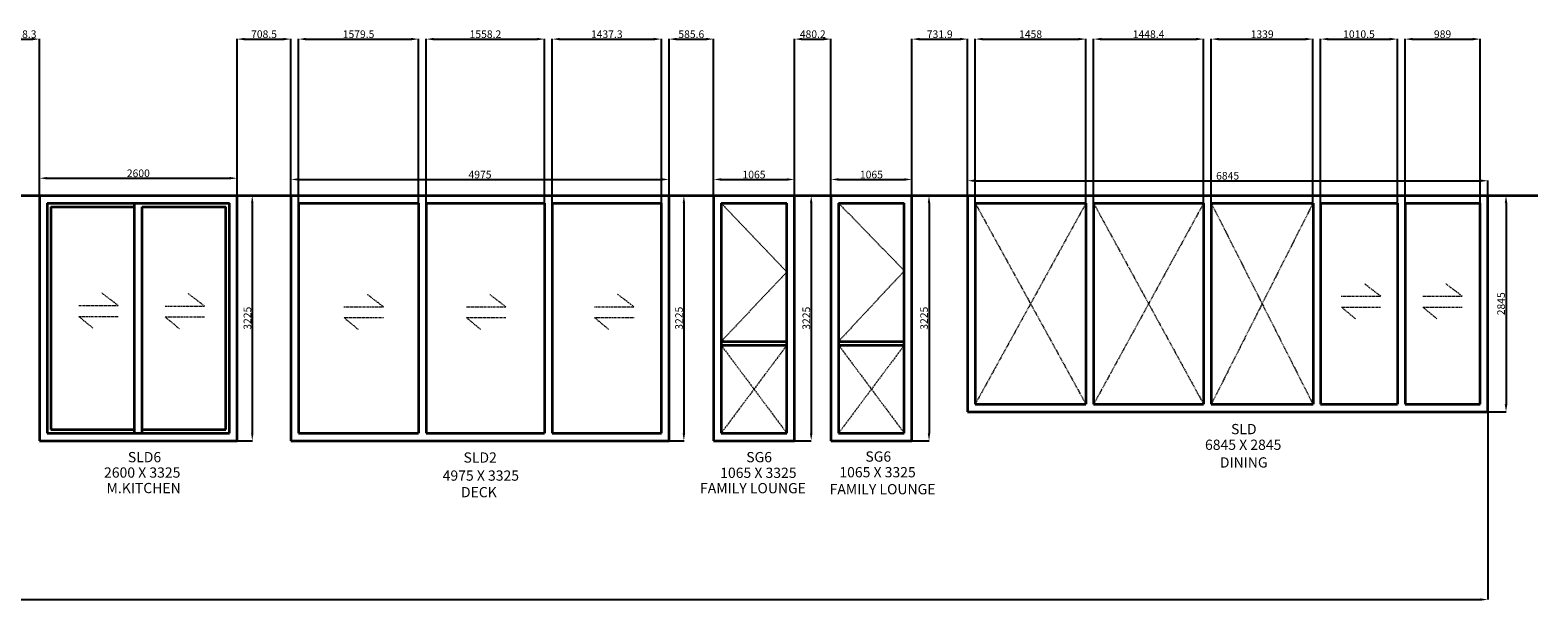
# Model space of a CAD drawing. Units: millimetres. Extents: x -850 to 42148, y -7352 to 4589.
# Tile 4 of 4: x 22310 to 42148, y -2915 to 4589. Entities that reach past the tile are written whole.
import ezdxf

# ---------------------------------------------------------------- set-up
doc = ezdxf.new("R2010")
doc.units = ezdxf.units.MM
doc.linetypes.add('DASHED', pattern=[19.05, 12.7, -6.35])
for name, color, linetype, lineweight in [('A-ANNO-DIMS', 2, 'Continuous', 18), ('A-ANNO-TEXT', 7, 'Continuous', 18), ('A-GLAZ', 4, 'Continuous', 35), ('A-GLAZ-OPNG', 4, 'DASHED', 18)]:
    doc.layers.add(name, color=color, linetype=linetype, lineweight=lineweight)
doc.styles.get("Standard").update_dxf_attribs({"font": 'arial.ttf'})
doc.dimstyles.new('ISO-25', dxfattribs={"dimtxt": 100, "dimasz": 100, "dimexe": 1.25, "dimexo": 0.625, "dimtad": 1, "dimtxsty": 'Standard', "dimcen": 2.5, "dimadec": 0, "dimazin": 0, "dimtfac": 1, "dimtmove": 0, "dimatfit": 3, "dimfxl": 1, "dimarcsym": 0})

# ---------------------------------------------------------------- blocks, each defined once
blk = doc.blocks.new('*D19')
at = {"layer": 'A-ANNO-DIMS', "color": 0, "lineweight": -2, "transparency": 16777216}
for p, q in [((22433, 2415), (22433, 2644)), ((22533, 2642), (24933, 2642)), ((25033, 2415), (25033, 2644))]:
    blk.add_line(p, q, dxfattribs=at)
at = {"layer": 'A-ANNO-DIMS', "color": 0, "lineweight": 30, "transparency": 16777216}
for points in [[(22533, 2659), (22533, 2626), (22433, 2642)], [(24933, 2659), (24933, 2626), (25033, 2642)]]:
    blk.add_solid(points, dxfattribs=at)
at = {"layer": 'Defpoints', "color": 0, "lineweight": 30, "transparency": 16777216}
for p in [(25033, 2642), (22433, 2414), (25033, 2414)]:
    blk.add_point(p, dxfattribs=at)
at = {"layer": 'A-ANNO-DIMS', "color": 0, "transparency": 16777216, "insert": (23733, 2694), "char_height": 100, "attachment_point": 5}
blk.add_mtext('2600', dxfattribs=at)
blk = doc.blocks.new('*D20')
at = {"layer": 'A-ANNO-DIMS', "color": 0, "lineweight": -2, "transparency": 16777216}
for p, q in [((25033, 2414), (25234, 2414)), ((25232, 2314), (25232, -711)), ((25033, -811), (25234, -811))]:
    blk.add_line(p, q, dxfattribs=at)
at = {"layer": 'A-ANNO-DIMS', "color": 0, "lineweight": 30, "transparency": 16777216}
for points in [[(25216, 2314), (25249, 2314), (25232, 2414)], [(25216, -711), (25249, -711), (25232, -811)]]:
    blk.add_solid(points, dxfattribs=at)
at = {"layer": 'Defpoints', "color": 0, "lineweight": 30, "transparency": 16777216}
for p in [(25033, 2414), (25033, -811), (25232, -811)]:
    blk.add_point(p, dxfattribs=at)
at = {"layer": 'A-ANNO-DIMS', "color": 0, "transparency": 16777216, "insert": (25181, 801), "char_height": 100, "attachment_point": 5, "rotation": 90}
blk.add_mtext('3225', dxfattribs=at)
blk = doc.blocks.new('*D21')
at = {"layer": 'A-ANNO-DIMS', "color": 0, "lineweight": -2, "transparency": 16777216}
for p, q in [((25741, 2415), (25741, 2627)), ((25841, 2626), (30616, 2626)), ((30716, 2415), (30716, 2627))]:
    blk.add_line(p, q, dxfattribs=at)
at = {"layer": 'A-ANNO-DIMS', "color": 0, "lineweight": 30, "transparency": 16777216}
for points in [[(25841, 2642), (25841, 2609), (25741, 2626)], [(30616, 2642), (30616, 2609), (30716, 2626)]]:
    blk.add_solid(points, dxfattribs=at)
at = {"layer": 'Defpoints', "color": 0, "lineweight": 30, "transparency": 16777216}
for p in [(30716, 2626), (25741, 2414), (30716, 2414)]:
    blk.add_point(p, dxfattribs=at)
at = {"layer": 'A-ANNO-DIMS', "color": 0, "transparency": 16777216, "insert": (28229, 2677), "char_height": 100, "attachment_point": 5}
blk.add_mtext('4975', dxfattribs=at)
blk = doc.blocks.new('*D22')
at = {"layer": 'A-ANNO-DIMS', "color": 0, "lineweight": -2, "transparency": 16777216}
for p, q in [((30717, 2414), (30913, 2414)), ((30911, 2314), (30911, -711)), ((30717, -811), (30913, -811))]:
    blk.add_line(p, q, dxfattribs=at)
at = {"layer": 'A-ANNO-DIMS', "color": 0, "lineweight": 30, "transparency": 16777216}
for points in [[(30895, 2314), (30928, 2314), (30911, 2414)], [(30895, -711), (30928, -711), (30911, -811)]]:
    blk.add_solid(points, dxfattribs=at)
at = {"layer": 'Defpoints', "color": 0, "lineweight": 30, "transparency": 16777216}
for p in [(30716, 2414), (30716, -811), (30911, -811)]:
    blk.add_point(p, dxfattribs=at)
at = {"layer": 'A-ANNO-DIMS', "color": 0, "transparency": 16777216, "insert": (30860, 801), "char_height": 100, "attachment_point": 5, "rotation": 90}
blk.add_mtext('3225', dxfattribs=at)
blk = doc.blocks.new('*D23')
at = {"layer": 'A-ANNO-DIMS', "color": 0, "lineweight": -2, "transparency": 16777216}
for p, q in [((31302, 2415), (31302, 2627)), ((31402, 2626), (32267, 2626)), ((32367, 2415), (32367, 2627))]:
    blk.add_line(p, q, dxfattribs=at)
at = {"layer": 'A-ANNO-DIMS', "color": 0, "lineweight": 30, "transparency": 16777216}
for points in [[(31402, 2642), (31402, 2609), (31302, 2626)], [(32267, 2642), (32267, 2609), (32367, 2626)]]:
    blk.add_solid(points, dxfattribs=at)
at = {"layer": 'Defpoints', "color": 0, "lineweight": 30, "transparency": 16777216}
for p in [(32367, 2626), (31302, 2414), (32367, 2414)]:
    blk.add_point(p, dxfattribs=at)
at = {"layer": 'A-ANNO-DIMS', "color": 0, "transparency": 16777216, "insert": (31834, 2677), "char_height": 100, "attachment_point": 5}
blk.add_mtext('1065', dxfattribs=at)
blk = doc.blocks.new('*D24')
at = {"layer": 'A-ANNO-DIMS', "color": 0, "lineweight": -2, "transparency": 16777216}
for p, q in [((32367, 2414), (32588, 2414)), ((32587, 2314), (32587, -711)), ((32367, -811), (32588, -811))]:
    blk.add_line(p, q, dxfattribs=at)
at = {"layer": 'A-ANNO-DIMS', "color": 0, "lineweight": 30, "transparency": 16777216}
for points in [[(32570, 2314), (32603, 2314), (32587, 2414)], [(32570, -711), (32603, -711), (32587, -811)]]:
    blk.add_solid(points, dxfattribs=at)
at = {"layer": 'Defpoints', "color": 0, "lineweight": 30, "transparency": 16777216}
for p in [(32367, 2414), (32367, -811), (32587, -811)]:
    blk.add_point(p, dxfattribs=at)
at = {"layer": 'A-ANNO-DIMS', "color": 0, "transparency": 16777216, "insert": (32535, 801), "char_height": 100, "attachment_point": 5, "rotation": 90}
blk.add_mtext('3225', dxfattribs=at)
blk = doc.blocks.new('*D25')
at = {"layer": 'A-ANNO-DIMS', "color": 0, "lineweight": -2, "transparency": 16777216}
for p, q in [((32847, 2415), (32847, 2627)), ((32947, 2626), (33812, 2626)), ((33912, 2415), (33912, 2627))]:
    blk.add_line(p, q, dxfattribs=at)
at = {"layer": 'A-ANNO-DIMS', "color": 0, "lineweight": 30, "transparency": 16777216}
for points in [[(32947, 2642), (32947, 2609), (32847, 2626)], [(33812, 2642), (33812, 2609), (33912, 2626)]]:
    blk.add_solid(points, dxfattribs=at)
at = {"layer": 'Defpoints', "color": 0, "lineweight": 30, "transparency": 16777216}
for p in [(33912, 2626), (32847, 2414), (33912, 2414)]:
    blk.add_point(p, dxfattribs=at)
at = {"layer": 'A-ANNO-DIMS', "color": 0, "transparency": 16777216, "insert": (33379, 2677), "char_height": 100, "attachment_point": 5}
blk.add_mtext('1065', dxfattribs=at)
blk = doc.blocks.new('*D26')
at = {"layer": 'A-ANNO-DIMS', "color": 0, "lineweight": -2, "transparency": 16777216}
for p, q in [((33912, 2414), (34138, 2414)), ((34137, 2314), (34137, -711)), ((33912, -811), (34138, -811))]:
    blk.add_line(p, q, dxfattribs=at)
at = {"layer": 'A-ANNO-DIMS', "color": 0, "lineweight": 30, "transparency": 16777216}
for points in [[(34120, 2314), (34153, 2314), (34137, 2414)], [(34120, -711), (34153, -711), (34137, -811)]]:
    blk.add_solid(points, dxfattribs=at)
at = {"layer": 'Defpoints', "color": 0, "lineweight": 30, "transparency": 16777216}
for p in [(33912, 2414), (33912, -811), (34137, -811)]:
    blk.add_point(p, dxfattribs=at)
at = {"layer": 'A-ANNO-DIMS', "color": 0, "transparency": 16777216, "insert": (34085, 801), "char_height": 100, "attachment_point": 5, "rotation": 90}
blk.add_mtext('3225', dxfattribs=at)
blk = doc.blocks.new('*D27')
at = {"layer": 'A-ANNO-DIMS', "color": 0, "lineweight": -2, "transparency": 16777216}
for p, q in [((34644, 2415), (34644, 2610)), ((34744, 2609), (41389, 2609)), ((41489, 2415), (41489, 2610))]:
    blk.add_line(p, q, dxfattribs=at)
at = {"layer": 'A-ANNO-DIMS', "color": 0, "lineweight": 30, "transparency": 16777216}
for points in [[(34744, 2626), (34744, 2592), (34644, 2609)], [(41389, 2626), (41389, 2592), (41489, 2609)]]:
    blk.add_solid(points, dxfattribs=at)
at = {"layer": 'Defpoints', "color": 0, "lineweight": 30, "transparency": 16777216}
for p in [(41489, 2609), (34644, 2414), (41489, 2414)]:
    blk.add_point(p, dxfattribs=at)
at = {"layer": 'A-ANNO-DIMS', "color": 0, "transparency": 16777216, "insert": (38066, 2661), "char_height": 100, "attachment_point": 5}
blk.add_mtext('6845', dxfattribs=at)
blk = doc.blocks.new('*D28')
at = {"layer": 'A-ANNO-DIMS', "color": 0, "lineweight": -2, "transparency": 16777216}
for p, q in [((41489, 2414), (41730, 2414)), ((41729, 2314), (41729, -331)), ((41489, -431), (41730, -431))]:
    blk.add_line(p, q, dxfattribs=at)
at = {"layer": 'A-ANNO-DIMS', "color": 0, "lineweight": 30, "transparency": 16777216}
for points in [[(41712, 2314), (41746, 2314), (41729, 2414)], [(41712, -331), (41746, -331), (41729, -431)]]:
    blk.add_solid(points, dxfattribs=at)
at = {"layer": 'Defpoints', "color": 0, "lineweight": 30, "transparency": 16777216}
for p in [(41489, 2414), (41489, -431), (41729, -431)]:
    blk.add_point(p, dxfattribs=at)
at = {"layer": 'A-ANNO-DIMS', "color": 0, "transparency": 16777216, "insert": (41677, 991), "char_height": 100, "attachment_point": 5, "rotation": 90}
blk.add_mtext('2845', dxfattribs=at)
blk = doc.blocks.new('SYM-SLIDE-ARROW')
for p, q in [((2602, 903), (2388, 1066)), ((2084, 903), (2602, 903)), ((2085, 760), (2604, 760)), ((2085, 760), (2269, 607))]:
    blk.add_line(p, q)
blk = doc.blocks.new('*D60')
at = {"layer": 'A-ANNO-DIMS', "color": 0, "lineweight": -2, "transparency": 16777216}
for p, q in [((41489, -432), (41489, -2900)), ((1325, -812), (1325, -2900)), ((1425, -2899), (41389, -2899))]:
    blk.add_line(p, q, dxfattribs=at)
at = {"layer": 'A-ANNO-DIMS', "color": 0, "lineweight": 30, "transparency": 16777216}
for points in [[(1425, -2882), (1425, -2915), (1325, -2899)], [(41389, -2882), (41389, -2915), (41489, -2899)]]:
    blk.add_solid(points, dxfattribs=at)
at = {"layer": 'Defpoints', "color": 0, "lineweight": 30, "transparency": 16777216}
for p in [(41489, -431), (1325, -811), (41489, -2899)]:
    blk.add_point(p, dxfattribs=at)
at = {"layer": 'A-ANNO-DIMS', "color": 0, "transparency": 16777216, "insert": (21407, -2847), "char_height": 100, "attachment_point": 5}
blk.add_mtext('40164', dxfattribs=at)
blk = doc.blocks.new('*D69')
at = {"layer": 'A-ANNO-DIMS', "color": 0, "lineweight": -2, "transparency": 16777216}
for p, q in [((22014, 2415), (22014, 4473)), ((22114, 4471), (22333, 4471)), ((22433, 2415), (22433, 4473))]:
    blk.add_line(p, q, dxfattribs=at)
at = {"layer": 'A-ANNO-DIMS', "color": 0, "lineweight": 30, "transparency": 16777216}
for points in [[(22114, 4488), (22114, 4455), (22014, 4471)], [(22333, 4488), (22333, 4455), (22433, 4471)]]:
    blk.add_solid(points, dxfattribs=at)
at = {"layer": 'Defpoints', "color": 0, "lineweight": 30, "transparency": 16777216}
for p in [(22433, 4471), (22014, 2414), (22433, 2414)]:
    blk.add_point(p, dxfattribs=at)
at = {"layer": 'A-ANNO-DIMS', "color": 0, "transparency": 16777216, "insert": (22223, 4523), "char_height": 100, "attachment_point": 5}
blk.add_mtext('418.3', dxfattribs=at)
blk = doc.blocks.new('*D70')
at = {"layer": 'A-ANNO-DIMS', "color": 0, "lineweight": -2, "transparency": 16777216}
for p, q in [((25033, 2415), (25033, 4473)), ((25133, 4471), (25641, 4471)), ((25741, 2415), (25741, 4473))]:
    blk.add_line(p, q, dxfattribs=at)
at = {"layer": 'A-ANNO-DIMS', "color": 0, "lineweight": 30, "transparency": 16777216}
for points in [[(25133, 4488), (25133, 4455), (25033, 4471)], [(25641, 4488), (25641, 4455), (25741, 4471)]]:
    blk.add_solid(points, dxfattribs=at)
at = {"layer": 'Defpoints', "color": 0, "lineweight": 30, "transparency": 16777216}
for p in [(25741, 4471), (25033, 2414), (25741, 2414)]:
    blk.add_point(p, dxfattribs=at)
at = {"layer": 'A-ANNO-DIMS', "color": 0, "transparency": 16777216, "insert": (25387, 4523), "char_height": 100, "attachment_point": 5}
blk.add_mtext('708.5', dxfattribs=at)
blk = doc.blocks.new('*D71')
at = {"layer": 'A-ANNO-DIMS', "color": 0, "lineweight": -2, "transparency": 16777216}
for p, q in [((30716, 2415), (30716, 4473)), ((30816, 4471), (31202, 4471)), ((31302, 2415), (31302, 4473))]:
    blk.add_line(p, q, dxfattribs=at)
at = {"layer": 'A-ANNO-DIMS', "color": 0, "lineweight": 30, "transparency": 16777216}
for points in [[(30816, 4488), (30816, 4455), (30716, 4471)], [(31202, 4488), (31202, 4455), (31302, 4471)]]:
    blk.add_solid(points, dxfattribs=at)
at = {"layer": 'Defpoints', "color": 0, "lineweight": 30, "transparency": 16777216}
for p in [(31302, 4471), (30716, 2414), (31302, 2414)]:
    blk.add_point(p, dxfattribs=at)
at = {"layer": 'A-ANNO-DIMS', "color": 0, "transparency": 16777216, "insert": (31009, 4523), "char_height": 100, "attachment_point": 5}
blk.add_mtext('585.6', dxfattribs=at)
blk = doc.blocks.new('*D72')
at = {"layer": 'A-ANNO-DIMS', "color": 0, "lineweight": -2, "transparency": 16777216}
for p, q in [((32367, 2415), (32367, 4473)), ((32467, 4471), (32747, 4471)), ((32847, 2415), (32847, 4473))]:
    blk.add_line(p, q, dxfattribs=at)
at = {"layer": 'A-ANNO-DIMS', "color": 0, "lineweight": 30, "transparency": 16777216}
for points in [[(32467, 4488), (32467, 4455), (32367, 4471)], [(32747, 4488), (32747, 4455), (32847, 4471)]]:
    blk.add_solid(points, dxfattribs=at)
at = {"layer": 'Defpoints', "color": 0, "lineweight": 30, "transparency": 16777216}
for p in [(32847, 4471), (32367, 2414), (32847, 2414)]:
    blk.add_point(p, dxfattribs=at)
at = {"layer": 'A-ANNO-DIMS', "color": 0, "transparency": 16777216, "insert": (32607, 4523), "char_height": 100, "attachment_point": 5}
blk.add_mtext('480.2', dxfattribs=at)
blk = doc.blocks.new('*D73')
at = {"layer": 'A-ANNO-DIMS', "color": 0, "lineweight": -2, "transparency": 16777216}
for p, q in [((33912, 2415), (33912, 4473)), ((34012, 4471), (34544, 4471)), ((34644, 2415), (34644, 4473))]:
    blk.add_line(p, q, dxfattribs=at)
at = {"layer": 'A-ANNO-DIMS', "color": 0, "lineweight": 30, "transparency": 16777216}
for points in [[(34012, 4488), (34012, 4455), (33912, 4471)], [(34544, 4488), (34544, 4455), (34644, 4471)]]:
    blk.add_solid(points, dxfattribs=at)
at = {"layer": 'Defpoints', "color": 0, "lineweight": 30, "transparency": 16777216}
for p in [(34644, 4471), (33912, 2414), (34644, 2414)]:
    blk.add_point(p, dxfattribs=at)
at = {"layer": 'A-ANNO-DIMS', "color": 0, "transparency": 16777216, "insert": (34278, 4523), "char_height": 100, "attachment_point": 5}
blk.add_mtext('731.9', dxfattribs=at)
blk = doc.blocks.new('*D75')
at = {"layer": 'A-ANNO-DIMS', "color": 0, "lineweight": -2, "transparency": 16777216}
for p, q in [((34744, 2315), (34744, 4473)), ((34844, 4471), (36102, 4471)), ((36202, 2315), (36202, 4473))]:
    blk.add_line(p, q, dxfattribs=at)
at = {"layer": 'A-ANNO-DIMS', "color": 0, "lineweight": 30, "transparency": 16777216}
for points in [[(34844, 4488), (34844, 4455), (34744, 4471)], [(36102, 4488), (36102, 4455), (36202, 4471)]]:
    blk.add_solid(points, dxfattribs=at)
at = {"layer": 'Defpoints', "color": 0, "lineweight": 30, "transparency": 16777216}
for p in [(36202, 4471), (34744, 2314), (36202, 2314)]:
    blk.add_point(p, dxfattribs=at)
at = {"layer": 'A-ANNO-DIMS', "color": 0, "transparency": 16777216, "insert": (35473, 4523), "char_height": 100, "attachment_point": 5}
blk.add_mtext('1458', dxfattribs=at)
blk = doc.blocks.new('*D76')
at = {"layer": 'A-ANNO-DIMS', "color": 0, "lineweight": -2, "transparency": 16777216}
for p, q in [((36302, 2315), (36302, 4473)), ((36402, 4471), (37650, 4471)), ((37750, 2315), (37750, 4473))]:
    blk.add_line(p, q, dxfattribs=at)
at = {"layer": 'A-ANNO-DIMS', "color": 0, "lineweight": 30, "transparency": 16777216}
for points in [[(36402, 4488), (36402, 4455), (36302, 4471)], [(37650, 4488), (37650, 4455), (37750, 4471)]]:
    blk.add_solid(points, dxfattribs=at)
at = {"layer": 'Defpoints', "color": 0, "lineweight": 30, "transparency": 16777216}
for p in [(37750, 4471), (36302, 2314), (37750, 2314)]:
    blk.add_point(p, dxfattribs=at)
at = {"layer": 'A-ANNO-DIMS', "color": 0, "transparency": 16777216, "insert": (37026, 4523), "char_height": 100, "attachment_point": 5}
blk.add_mtext('1448.4', dxfattribs=at)
blk = doc.blocks.new('*D77')
at = {"layer": 'A-ANNO-DIMS', "color": 0, "lineweight": -2, "transparency": 16777216}
for p, q in [((37850, 2315), (37850, 4473)), ((37950, 4471), (39089, 4471)), ((39189, 2315), (39189, 4473))]:
    blk.add_line(p, q, dxfattribs=at)
at = {"layer": 'A-ANNO-DIMS', "color": 0, "lineweight": 30, "transparency": 16777216}
for points in [[(37950, 4488), (37950, 4455), (37850, 4471)], [(39089, 4488), (39089, 4455), (39189, 4471)]]:
    blk.add_solid(points, dxfattribs=at)
at = {"layer": 'Defpoints', "color": 0, "lineweight": 30, "transparency": 16777216}
for p in [(39189, 4471), (37850, 2314), (39189, 2314)]:
    blk.add_point(p, dxfattribs=at)
at = {"layer": 'A-ANNO-DIMS', "color": 0, "transparency": 16777216, "insert": (38520, 4523), "char_height": 100, "attachment_point": 5}
blk.add_mtext('1339', dxfattribs=at)
blk = doc.blocks.new('*D78')
at = {"layer": 'A-ANNO-DIMS', "color": 0, "lineweight": -2, "transparency": 16777216}
for p, q in [((39289, 2315), (39289, 4473)), ((39389, 4471), (40200, 4471)), ((40300, 2315), (40300, 4473))]:
    blk.add_line(p, q, dxfattribs=at)
at = {"layer": 'A-ANNO-DIMS', "color": 0, "lineweight": 30, "transparency": 16777216}
for points in [[(39389, 4488), (39389, 4455), (39289, 4471)], [(40200, 4488), (40200, 4455), (40300, 4471)]]:
    blk.add_solid(points, dxfattribs=at)
at = {"layer": 'Defpoints', "color": 0, "lineweight": 30, "transparency": 16777216}
for p in [(40300, 4471), (39289, 2314), (40300, 2314)]:
    blk.add_point(p, dxfattribs=at)
at = {"layer": 'A-ANNO-DIMS', "color": 0, "transparency": 16777216, "insert": (39794, 4523), "char_height": 100, "attachment_point": 5}
blk.add_mtext('1010.5', dxfattribs=at)
blk = doc.blocks.new('*D79')
at = {"layer": 'A-ANNO-DIMS', "color": 0, "lineweight": -2, "transparency": 16777216}
for p, q in [((40400, 2315), (40400, 4473)), ((40500, 4471), (41289, 4471)), ((41389, 2315), (41389, 4473))]:
    blk.add_line(p, q, dxfattribs=at)
at = {"layer": 'A-ANNO-DIMS', "color": 0, "lineweight": 30, "transparency": 16777216}
for points in [[(40500, 4488), (40500, 4455), (40400, 4471)], [(41289, 4488), (41289, 4455), (41389, 4471)]]:
    blk.add_solid(points, dxfattribs=at)
at = {"layer": 'Defpoints', "color": 0, "lineweight": 30, "transparency": 16777216}
for p in [(41389, 4471), (40400, 2314), (41389, 2314)]:
    blk.add_point(p, dxfattribs=at)
at = {"layer": 'A-ANNO-DIMS', "color": 0, "transparency": 16777216, "insert": (40894, 4523), "char_height": 100, "attachment_point": 5}
blk.add_mtext('989', dxfattribs=at)
blk = doc.blocks.new('*D80')
at = {"layer": 'A-ANNO-DIMS', "color": 0, "lineweight": -2, "transparency": 16777216}
for p, q in [((25841, 2315), (25841, 4473)), ((25941, 4471), (27321, 4471)), ((27421, 2315), (27421, 4473))]:
    blk.add_line(p, q, dxfattribs=at)
at = {"layer": 'A-ANNO-DIMS', "color": 0, "lineweight": 30, "transparency": 16777216}
for points in [[(25941, 4488), (25941, 4455), (25841, 4471)], [(27321, 4488), (27321, 4455), (27421, 4471)]]:
    blk.add_solid(points, dxfattribs=at)
at = {"layer": 'Defpoints', "color": 0, "lineweight": 30, "transparency": 16777216}
for p in [(27421, 4471), (25841, 2314), (27421, 2314)]:
    blk.add_point(p, dxfattribs=at)
at = {"layer": 'A-ANNO-DIMS', "color": 0, "transparency": 16777216, "insert": (26631, 4523), "char_height": 100, "attachment_point": 5}
blk.add_mtext('1579.5', dxfattribs=at)
blk = doc.blocks.new('*D81')
at = {"layer": 'A-ANNO-DIMS', "color": 0, "lineweight": -2, "transparency": 16777216}
for p, q in [((27521, 2315), (27521, 4473)), ((27621, 4471), (28979, 4471)), ((29079, 2315), (29079, 4473))]:
    blk.add_line(p, q, dxfattribs=at)
at = {"layer": 'A-ANNO-DIMS', "color": 0, "lineweight": 30, "transparency": 16777216}
for points in [[(27621, 4488), (27621, 4455), (27521, 4471)], [(28979, 4488), (28979, 4455), (29079, 4471)]]:
    blk.add_solid(points, dxfattribs=at)
at = {"layer": 'Defpoints', "color": 0, "lineweight": 30, "transparency": 16777216}
for p in [(29079, 4471), (27521, 2314), (29079, 2314)]:
    blk.add_point(p, dxfattribs=at)
at = {"layer": 'A-ANNO-DIMS', "color": 0, "transparency": 16777216, "insert": (28300, 4523), "char_height": 100, "attachment_point": 5}
blk.add_mtext('1558.2', dxfattribs=at)
blk = doc.blocks.new('*D82')
at = {"layer": 'A-ANNO-DIMS', "color": 0, "lineweight": -2, "transparency": 16777216}
for p, q in [((29179, 2315), (29179, 4473)), ((29279, 4471), (30516, 4471)), ((30616, 2315), (30616, 4473))]:
    blk.add_line(p, q, dxfattribs=at)
at = {"layer": 'A-ANNO-DIMS', "color": 0, "lineweight": 30, "transparency": 16777216}
for points in [[(29279, 4488), (29279, 4455), (29179, 4471)], [(30516, 4488), (30516, 4455), (30616, 4471)]]:
    blk.add_solid(points, dxfattribs=at)
at = {"layer": 'Defpoints', "color": 0, "lineweight": 30, "transparency": 16777216}
for p in [(30616, 4471), (29179, 2314), (30616, 2314)]:
    blk.add_point(p, dxfattribs=at)
at = {"layer": 'A-ANNO-DIMS', "color": 0, "transparency": 16777216, "insert": (29897, 4523), "char_height": 100, "attachment_point": 5}
blk.add_mtext('1437.3', dxfattribs=at)

msp = doc.modelspace()

# ---------------------------------------------------------------- linework, layer by layer
at = {"layer": 'A-GLAZ'}
for p, q in [((15219.457, 2413.876), (42147.613, 2413.876)), ((22432.638, 2413.876), (22432.638, -811.124)), ((25032.638, -811.124), (25032.638, 2413.876)), ((25741.095, 2413.876), (25741.095, -811.124)), ((30716.095, -811.124), (30716.095, 2413.876)), ((31301.669, 2413.876), (31301.669, -811.124)), ((32366.669, -811.124), (32366.669, 2413.876)), ((32846.844, 2413.876), (32846.844, -811.124)), ((33911.844, -811.124), (33911.844, 2413.876)), ((34643.766, 2413.876), (34643.766, -431.124)), ((41488.766, -431.124), (41488.766, 2413.876)), ((22532.638, 2313.876), (24932.638, 2313.876)), ((22532.638, 2313.876), (22532.638, -711.124)), ((22582.638, 2263.876), (22582.638, -661.124)), ((22582.638, 2263.876), (23682.638, 2263.876)), ((23682.638, -711.124), (23682.638, 2313.876)), ((23782.638, -711.124), (23782.638, 2263.876)), ((23782.638, 2263.876), (24882.638, 2263.876)), ((24882.638, -661.124), (24882.638, 2263.876)), ((24932.638, -711.124), (24932.638, 2313.876)), ((25841.095, 2313.876), (27420.566, 2313.876)), ((25841.095, 2313.876), (25841.095, -711.124)), ((27420.566, 2313.876), (27420.566, -711.124)), ((27520.566, 2313.876), (27520.566, -711.124)), ((27520.566, 2313.876), (29078.754, 2313.876)), ((29078.754, 2313.876), (29078.754, -711.124)), ((29178.754, 2313.876), (29178.754, -711.124)), ((29178.754, 2313.876), (30616.095, 2313.876)), ((30616.095, -711.124), (30616.095, 2313.876)), ((31401.669, 2313.876), (32266.669, 2313.876)), ((31401.669, 2313.876), (31401.669, -711.124)), ((32266.669, -711.124), (32266.669, 2313.876)), ((32946.844, 2313.876), (32946.844, -711.124)), ((32946.844, 2313.876), (33811.844, 2313.876)), ((33811.844, -711.124), (33811.844, 2313.876)), ((34743.766, 2313.876), (34743.766, -331.124)), ((34743.766, 2313.876), (36201.908, 2313.876)), ((36201.908, 2313.876), (36201.908, -331.124)), ((36301.908, 2313.876), (36301.908, -331.124)), ((36301.908, 2313.876), (37750.325, 2313.876)), ((37750.325, 2313.876), (37750.325, -331.124)), ((37850.325, 2313.876), (37850.325, -331.124)), ((37850.325, 2313.876), (39189.258, 2313.876)), ((39189.258, 2313.876), (39189.258, -331.124)), ((39289.258, 2313.876), (39289.258, -331.124)), ((39289.258, 2313.876), (40299.738, 2313.876)), ((40299.738, 2313.876), (40299.738, -331.124)), ((40399.738, 2313.876), (40399.738, -331.124)), ((40399.738, 2313.876), (41388.766, 2313.876)), ((41388.766, -331.124), (41388.766, 2313.876)), ((31401.669, 496.763), (32266.669, 496.763)), ((31401.669, 446.763), (32266.669, 446.763)), ((32946.844, 496.763), (33811.844, 496.763)), ((32946.844, 446.763), (33811.844, 446.763)), ((34743.766, -331.124), (36201.908, -331.124)), ((36301.908, -331.124), (37750.325, -331.124)), ((37850.325, -331.124), (39189.258, -331.124)), ((39289.258, -331.124), (40299.738, -331.124)), ((40399.738, -331.124), (41388.766, -331.124)), ((34643.766, -431.124), (41488.766, -431.124)), ((22532.638, -711.124), (24932.638, -711.124)), ((22582.638, -661.124), (23682.638, -661.124)), ((23782.638, -661.124), (24882.638, -661.124)), ((25841.095, -711.124), (27420.566, -711.124)), ((27520.566, -711.124), (29078.754, -711.124)), ((29178.754, -711.124), (30616.095, -711.124)), ((31401.669, -711.124), (32266.669, -711.124)), ((32946.844, -711.124), (33811.844, -711.124)), ((22432.638, -811.124), (25032.638, -811.124)), ((25741.095, -811.124), (30716.095, -811.124)), ((31301.669, -811.124), (32366.669, -811.124)), ((32846.844, -811.124), (33911.844, -811.124))]:
    msp.add_line(p, q, dxfattribs=at)
at = {"layer": 'A-GLAZ-OPNG'}
for p, q in [((31401.669, 2313.876), (32266.669, 1407.83)), ((32946.844, 2313.876), (33811.844, 1424.913)), ((34743.766, 2313.876), (36201.908, -331.124)), ((36201.908, 2313.876), (34743.766, -331.124)), ((36301.908, 2313.876), (37750.325, -331.124)), ((37750.325, 2313.876), (36301.908, -331.124)), ((37850.325, 2313.876), (39189.258, -331.124)), ((39189.258, 2313.876), (37850.325, -331.124)), ((32266.669, 1407.83), (31401.669, 496.763)), ((33811.844, 1424.913), (32946.844, 496.763)), ((31401.669, 446.763), (32266.669, -711.124)), ((32266.669, 446.763), (31401.669, -711.124)), ((32946.844, 446.763), (33811.844, -711.124)), ((33811.844, 446.763), (32946.844, -711.124))]:
    msp.add_line(p, q, dxfattribs=at)

# ---------------------------------------------------------------- block references
for p in [(37477.561, 188.014), (38549.338, 188.014), (20865.848, 65.004), (22001.521, 58.408), (24354.924, 48.946), (25965.905, 48.946), (27652.064, 48.946)]:
    msp.add_blockref('SYM-SLIDE-ARROW', p, dxfattribs=at)

# ---------------------------------------------------------------- texts
at = {"layer": 'A-ANNO-TEXT'}
for s, height, p in [('SLD', 134.8889, (38110.859, -724.457)), ('6845 X 2845', 134.88886, (37768.085, -930.294)), ('SLD6', 134.8889, (23595.216, -1093.156)), ('SLD2', 134.8889, (28011.861, -1098.41)), ('SG6', 134.8889, (31732.015, -1093.156)), ('SG6', 134.8889, (33299.837, -1085.573)), ('2600 X 3325', 134.88886, (23281.786, -1295.736)), ('1065 X 3325', 134.88886, (31389.242, -1298.993)), ('1065 X 3325', 134.88886, (32957.063, -1291.41)), ('DINING', 134.8889, (37963.612, -1162.82)), ('M.KITCHEN', 134.8889, (23314.757, -1499.944)), ('4975 X 3325', 134.88886, (27737.454, -1335.769)), ('FAMILY LOUNGE', 134.88886, (31123.991, -1501.182)), ('FAMILY LOUNGE', 134.88886, (32829.121, -1514.704)), ('DECK', 134.8889, (27978.259, -1553.742))]:
    msp.add_text(s, height=height, dxfattribs=at).set_placement(p)

# ---------------------------------------------------------------- dimensions: what is measured, and where the dimension line sits
at = {"layer": 'A-ANNO-DIMS'}
for base, p1, p2, override, picture, middle in [((22432.638, 4471.376), (22014.328, 2413.876), (22432.638, 2413.876), {"dimdec": 1, "dimlfac": 1, "dimrnd": 0, "dimzin": 0, "dimdsep": 46, "dimlunit": 2}, '*D69', (22223.483, 4523.092)), ((25741.095, 4471.376), (25032.638, 2413.876), (25741.095, 2413.876), {"dimdec": 1, "dimlfac": 1, "dimrnd": 0, "dimzin": 0, "dimdsep": 46, "dimlunit": 2}, '*D70', (25386.867, 4523.058)), ((27420.566, 4471.376), (25841.095, 2313.876), (27420.566, 2313.876), {"dimdec": 1, "dimlfac": 1, "dimrnd": 0, "dimzin": 0, "dimdsep": 46, "dimlunit": 2}, '*D80', (26630.83, 4523.058)), ((29078.754, 4471.376), (27520.566, 2313.876), (29078.754, 2313.876), {"dimdec": 1, "dimlfac": 1, "dimrnd": 0, "dimzin": 0, "dimdsep": 46, "dimlunit": 2}, '*D81', (28299.66, 4523.058)), ((30616.095, 4471.376), (29178.754, 2313.876), (30616.095, 2313.876), {"dimdec": 1, "dimlfac": 1, "dimrnd": 0, "dimzin": 0, "dimdsep": 46, "dimlunit": 2}, '*D82', (29897.424, 4523.092)), ((31301.669, 4471.376), (30716.095, 2413.876), (31301.669, 2413.876), {"dimdec": 1, "dimlfac": 1, "dimrnd": 0, "dimzin": 0, "dimdsep": 46, "dimlunit": 2}, '*D71', (31008.882, 4523.058)), ((32846.844, 4471.376), (32366.669, 2413.876), (32846.844, 2413.876), {"dimdec": 1, "dimlfac": 1, "dimrnd": 0, "dimzin": 0, "dimdsep": 46, "dimlunit": 2}, '*D72', (32606.757, 4523.058)), ((34643.766, 4471.376), (33911.844, 2413.876), (34643.766, 2413.876), {"dimdec": 1, "dimlfac": 1, "dimrnd": 0, "dimzin": 0, "dimdsep": 46, "dimlunit": 2}, '*D73', (34277.805, 4523.092)), ((36201.908, 4471.376), (34743.766, 2313.876), (36201.908, 2313.876), {"dimdec": 0, "dimlfac": 1, "dimrnd": 0, "dimzin": 0, "dimdsep": 46, "dimlunit": 2}, '*D75', (35472.837, 4523.058)), ((37750.325, 4471.376), (36301.908, 2313.876), (37750.325, 2313.876), {"dimdec": 1, "dimlfac": 1, "dimrnd": 0, "dimzin": 0, "dimdsep": 46, "dimlunit": 2}, '*D76', (37026.117, 4523.058)), ((39189.258, 4471.376), (37850.325, 2313.876), (39189.258, 2313.876), {"dimdec": 0, "dimlfac": 1, "dimrnd": 0, "dimzin": 0, "dimdsep": 46, "dimlunit": 2}, '*D77', (38519.791, 4523.092)), ((40299.738, 4471.376), (39289.258, 2313.876), (40299.738, 2313.876), {"dimdec": 1, "dimlfac": 1, "dimrnd": 0, "dimzin": 0, "dimdsep": 46, "dimlunit": 2}, '*D78', (39794.498, 4523.058)), ((41388.766, 4471.376), (40399.738, 2313.876), (41388.766, 2313.876), {"dimdec": 0, "dimlfac": 1, "dimrnd": 0, "dimzin": 0, "dimdsep": 46, "dimlunit": 2}, '*D79', (40894.252, 4523.058)), ((25032.638, 2642.346), (22432.638, 2413.876), (25032.638, 2413.876), {"dimclrd": 0, "dimclre": 0, "dimclrt": 0}, '*D19', (23732.638, 2694.028)), ((30716.095, 2625.679), (25741.095, 2413.876), (30716.095, 2413.876), {"dimclrd": 0, "dimclre": 0, "dimclrt": 0}, '*D21', (28228.595, 2677.361)), ((32366.669, 2625.679), (31301.669, 2413.876), (32366.669, 2413.876), {"dimclrd": 0, "dimclre": 0, "dimclrt": 0}, '*D23', (31834.169, 2677.361)), ((33911.844, 2625.679), (32846.844, 2413.876), (33911.844, 2413.876), {"dimclrd": 0, "dimclre": 0, "dimclrt": 0}, '*D25', (33379.344, 2677.361)), ((41488.766, 2609.012), (34643.766, 2413.876), (41488.766, 2413.876), {"dimclrd": 0, "dimclre": 0, "dimclrt": 0}, '*D27', (38066.266, 2660.695)), ((41488.766, -2898.624), (1325.061, -811.124), (41488.766, -431.124), {"dimdec": 0, "dimlfac": 1, "dimrnd": 0, "dimzin": 0, "dimdsep": 46, "dimlunit": 2}, '*D60', (21406.913, -2846.942))]:
    dim = msp.add_linear_dim(base=base, p1=p1, p2=p2, dimstyle='ISO-25', override=override, dxfattribs=at)
    dim.commit()
    dim.dimension.update_dxf_attribs({"geometry": picture, "text_midpoint": middle})
for base, p1, p2, picture, middle in [((25232.416, -811.124), (25032.638, 2413.876), (25032.638, -811.124), '*D20', (25180.699, 801.376)), ((30911.416, -811.124), (30716.095, 2413.876), (30716.095, -811.124), '*D22', (30859.7, 801.376)), ((32586.62, -811.124), (32366.669, 2413.876), (32366.669, -811.124), '*D24', (32534.903, 801.376)), ((34136.637, -811.124), (33911.844, 2413.876), (33911.844, -811.124), '*D26', (34084.921, 801.376)), ((41728.99, -431.124), (41488.766, 2413.876), (41488.766, -431.124), '*D28', (41677.308, 991.376))]:
    dim = msp.add_linear_dim(base=base, p1=p1, p2=p2, angle=90, dimstyle='ISO-25', override={"dimclrd": 0, "dimclre": 0, "dimclrt": 0}, dxfattribs=at)
    dim.commit()
    dim.dimension.update_dxf_attribs({"geometry": picture, "text_midpoint": middle})

doc.saveas('drawing.dxf')
